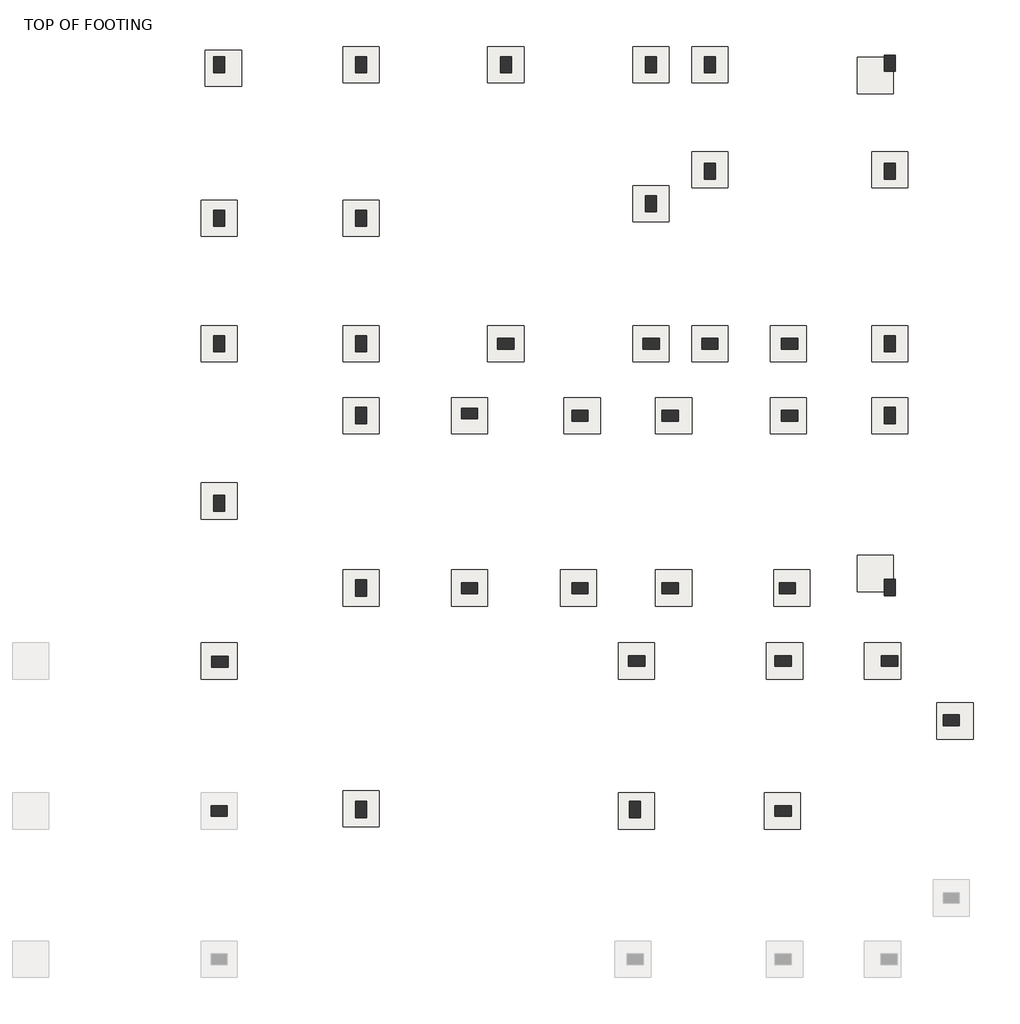
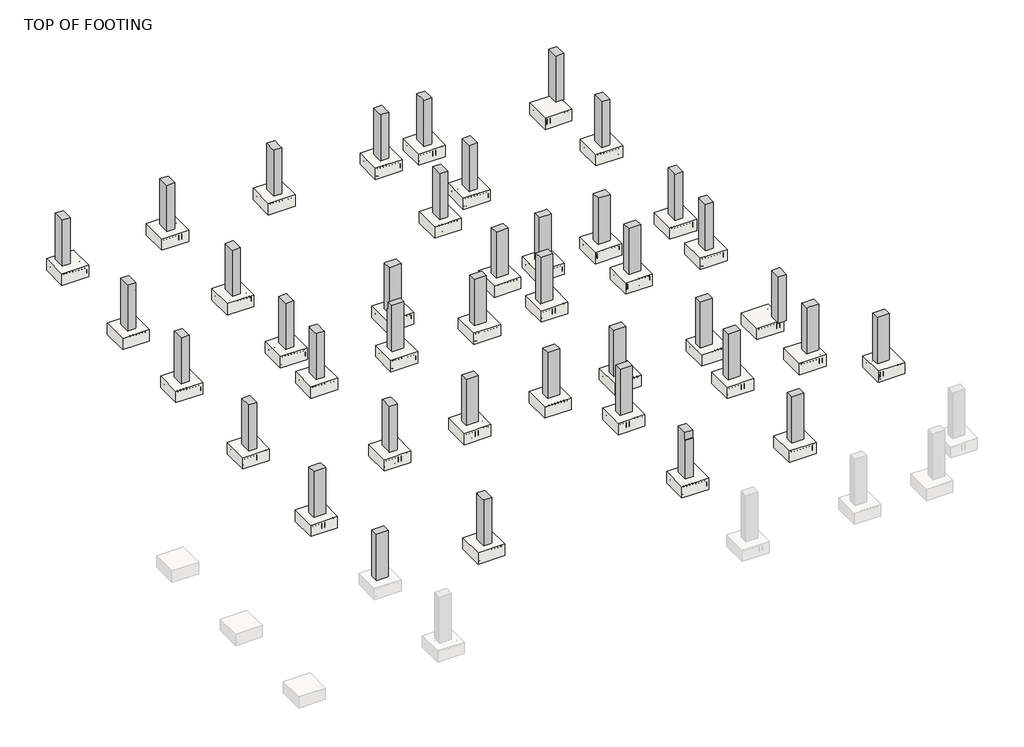
# One storey, part 2 of 20: 40 columns, 39 slabs.
"""IFC4 building model written with IfcOpenShell, lengths in millimetres."""

from ifc_helpers import new_model, si_unit, frame, origin, place, context, project, spatial, polyline, outline, extrude, faceted_brep, transform, mapped, element, save
from components import m_footing_rectangular_4c97ae35

model = new_model("IFC4")

# Units and contexts
model_context = context("Model", 3, world=origin())
ifc_project = project(units=[si_unit("LENGTHUNIT", "METRE", prefix="MILLI")], contexts=[model_context])

# Site, building, storey
site = spatial("IfcSite", under=ifc_project)
building = spatial("IfcBuilding", under=site)
storey = spatial("IfcBuildingStorey", under=building, Name="TOP OF FOOTING", Elevation=-1828.8)

# Columns
placement = place(None, origin())
element("IfcColumn", 1, ObjectType="M_Concrete-Rectangular-Column : 300 x 450mm", at=placement, inside=storey, context=model_context, shape_type="SweptSolid", body=[
    extrude(outline(polyline([(-5591.7865686, 21912.8349362), (-5591.7865686, 21462.8349362), (-5891.7865686, 21462.8349362), (-5891.7865686, 21912.8349362), (-5591.7865686, 21912.8349362)])), frame((0.0, 0.0, -1828.8), z_axis=(0.0, 0.0, 1.0), x_axis=(1.0, 0.0, 0.0)), (0.0, 0.0, 1.0), 1828.8),
])
element("IfcColumn", 2, ObjectType="M_Concrete-Rectangular-Column : 300 x 450mm", at=placement, inside=storey, context=model_context, shape_type="Brep", body=[
    faceted_brep([(-1671.7865686, 21912.8349362, -1828.8), (-1671.7865686, 21462.8349362, -1828.8), (-1971.7865686, 21462.8349362, -1828.8), (-1971.7865686, 21912.8349362, -1828.8), (-1671.7865686, 21912.8349362, 0.0), (-1671.7865686, 21537.8349362, 0.0), (-1671.7865686, 21462.8349362, 0.0), (-1671.7865686, 21462.8349362, -300.0), (-1971.7865686, 21462.8349362, 0.0), (-1971.7865686, 21462.8349362, -300.0), (-1971.7865686, 21912.8349362, 0.0)], [[[0, 1, 2, 3]], [[1, 0, 4, 5, 6, 7]], [[2, 1, 7, 6, 8, 9]], [[3, 2, 9, 8, 10]], [[0, 3, 10, 4]], [[8, 6, 5, 4, 10]]]),
])
element("IfcColumn", 3, ObjectType="M_Concrete-Rectangular-Column : 300 x 450mm", at=placement, inside=storey, context=model_context, shape_type="Brep", body=[
    faceted_brep([(2324.7296816, 21912.8349362, -1828.8), (2324.7296816, 21462.8349362, -1828.8), (2024.7296816, 21462.8349362, -1828.8), (2024.7296816, 21912.8349362, -1828.8), (2324.7296816, 21912.8349362, 0.0), (2324.7296816, 21537.8349362, 0.0), (2324.7296816, 21462.8349362, 0.0), (2324.7296816, 21462.8349362, -300.0), (2024.7296816, 21462.8349362, 0.0), (2024.7296816, 21462.8349362, -300.0), (2024.7296816, 21537.8349362, 0.0), (2024.7296816, 21912.8349362, 0.0)], [[[0, 1, 2, 3]], [[1, 0, 4, 5, 6, 7]], [[2, 1, 7, 6, 8, 9]], [[3, 2, 9, 8, 10, 11]], [[0, 3, 11, 4]], [[8, 6, 5, 4, 11, 10]]]),
])
element("IfcColumn", 4, ObjectType="M_Concrete-Rectangular-Column : 300 x 450mm", at=placement, inside=storey, context=model_context, shape_type="Brep", body=[
    faceted_brep([(6332.5248054, 21912.8349362, -1828.8), (6332.5248054, 21462.8349362, -1828.8), (6032.5248054, 21462.8349362, -1828.8), (6032.5248054, 21912.8349362, -1828.8), (6332.5248054, 21912.8349362, 0.0), (6332.5248054, 21537.8349362, 0.0), (6332.5248054, 21462.8349362, 0.0), (6332.5248054, 21462.8349362, -300.0), (6032.5248054, 21462.8349362, 0.0), (6032.5248054, 21462.8349362, -300.0), (6032.5248054, 21537.8349362, 0.0), (6032.5248054, 21912.8349362, 0.0)], [[[0, 1, 2, 3]], [[1, 0, 4, 5, 6, 7]], [[2, 1, 7, 6, 8, 9]], [[3, 2, 9, 8, 10, 11]], [[0, 3, 11, 4]], [[8, 6, 5, 4, 11, 10]]]),
])
element("IfcColumn", 5, ObjectType="M_Concrete-Rectangular-Column : 300 x 450mm", at=placement, inside=storey, context=model_context, shape_type="Brep", body=[
    faceted_brep([(7956.8679014, 21912.8349362, -1828.8), (7956.8679014, 21462.8349362, -1828.8), (7656.8679014, 21462.8349362, -1828.8), (7656.8679014, 21912.8349362, -1828.8), (7956.8679014, 21912.8349362, 0.0), (7956.8679014, 21537.8349362, 0.0), (7956.8679014, 21462.8349362, 0.0), (7956.8679014, 21462.8349362, -300.0), (7656.8679014, 21462.8349362, 0.0), (7656.8679014, 21462.8349362, -300.0), (7656.8679014, 21537.8349362, 0.0), (7656.8679014, 21912.8349362, 0.0)], [[[0, 1, 2, 3]], [[1, 0, 4, 5, 6, 7]], [[2, 1, 7, 6, 8, 9]], [[3, 2, 9, 8, 10, 11]], [[0, 3, 11, 4]], [[8, 6, 5, 4, 11, 10]]]),
])
element("IfcColumn", 6, ObjectType="M_Concrete-Rectangular-Column : 300 x 450mm", at=placement, inside=storey, context=model_context, shape_type="Brep", body=[
    faceted_brep([(12919.1163908, 21952.8349362, -1828.8), (12919.1163908, 21502.8349362, -1828.8), (12619.1163908, 21502.8349362, -1828.8), (12619.1163908, 21952.8349362, -1828.8), (12919.1163908, 21952.8349362, 0.0), (12919.1163908, 21502.8349362, 0.0), (12619.1163908, 21502.8349362, 0.0), (12619.1163908, 21502.8349362, -300.0), (12619.1163908, 21537.8349362, 0.0), (12619.1163908, 21952.8349362, 0.0)], [[[0, 1, 2, 3]], [[1, 0, 4, 5]], [[2, 1, 5, 6, 7]], [[3, 2, 7, 6, 8, 9]], [[0, 3, 9, 4]], [[5, 4, 9, 8, 6]]]),
])
element("IfcColumn", 7, ObjectType="M_Concrete-Rectangular-Column : 300 x 450mm", at=placement, inside=storey, context=model_context, shape_type="Brep", body=[
    faceted_brep([(12919.1163908, 18974.7148651, -1828.8), (12919.1163908, 18524.7148651, -1828.8), (12619.1163908, 18524.7148651, -1828.8), (12619.1163908, 18974.7148651, -1828.8), (12919.1163908, 18974.7148651, 0.0), (12919.1163908, 18524.7148651, 0.0), (12619.1163908, 18524.7148651, 0.0), (12619.1163908, 18524.7148651, -300.0), (12619.1163908, 18974.7148651, 0.0), (12619.1163908, 18974.7148651, -300.0)], [[[0, 1, 2, 3]], [[1, 0, 4, 5]], [[2, 1, 5, 6, 7]], [[3, 2, 7, 6, 8, 9]], [[0, 3, 9, 8, 4]], [[5, 4, 8, 6]]]),
])
element("IfcColumn", 8, ObjectType="M_Concrete-Rectangular-Column : 300 x 450mm", at=placement, inside=storey, context=model_context, shape_type="Brep", body=[
    faceted_brep([(7956.8679014, 18974.7148651, -1828.8), (7956.8679014, 18524.7148651, -1828.8), (7656.8679014, 18524.7148651, -1828.8), (7656.8679014, 18974.7148651, -1828.8), (7956.8679014, 18974.7148651, -300.0), (7956.8679014, 18974.7148651, 0.0), (7956.8679014, 18524.7148651, 0.0), (7956.8679014, 18524.7148651, -300.0), (7656.8679014, 18524.7148651, 0.0), (7656.8679014, 18524.7148651, -300.0), (7656.8679014, 18974.7148651, 0.0), (7656.8679014, 18974.7148651, -300.0)], [[[0, 1, 2, 3]], [[1, 0, 4, 5, 6, 7]], [[2, 1, 7, 6, 8, 9]], [[3, 2, 9, 8, 10, 11]], [[0, 3, 11, 10, 5, 4]], [[6, 5, 10, 8]]]),
])
element("IfcColumn", 9, ObjectType="M_Concrete-Rectangular-Column : 300 x 450mm", at=placement, inside=storey, context=model_context, shape_type="Brep", body=[
    faceted_brep([(6332.5248054, 18074.7148651, -1828.8), (6332.5248054, 17624.7148651, -1828.8), (6032.5248054, 17624.7148651, -1828.8), (6032.5248054, 18074.7148651, -1828.8), (6332.5248054, 18074.7148651, -300.0), (6332.5248054, 18074.7148651, 0.0), (6332.5248054, 17624.7148651, 0.0), (6332.5248054, 17624.7148651, -300.0), (6032.5248054, 17624.7148651, 0.0), (6032.5248054, 17624.7148651, -300.0), (6032.5248054, 18074.7148651, 0.0), (6032.5248054, 18074.7148651, -300.0)], [[[0, 1, 2, 3]], [[1, 0, 4, 5, 6, 7]], [[2, 1, 7, 6, 8, 9]], [[3, 2, 9, 8, 10, 11]], [[0, 3, 11, 10, 5, 4]], [[6, 5, 10, 8]]]),
])
element("IfcColumn", 10, ObjectType="M_Concrete-Rectangular-Column : 300 x 450mm", at=placement, inside=storey, context=model_context, shape_type="Brep", body=[
    faceted_brep([(-1671.7865686, 17674.7148651, -1828.8), (-1671.7865686, 17224.7148651, -1828.8), (-1971.7865686, 17224.7148651, -1828.8), (-1971.7865686, 17674.7148651, -1828.8), (-1671.7865686, 17674.7148651, -300.0), (-1671.7865686, 17674.7148651, 0.0), (-1671.7865686, 17224.7148651, 0.0), (-1671.7865686, 17224.7148651, -300.0), (-1971.7865686, 17224.7148651, 0.0), (-1971.7865686, 17224.7148651, -300.0), (-1971.7865686, 17674.7148651, 0.0), (-1971.7865686, 17674.7148651, -300.0)], [[[0, 1, 2, 3]], [[1, 0, 4, 5, 6, 7]], [[2, 1, 7, 6, 8, 9]], [[3, 2, 9, 8, 10, 11]], [[0, 3, 11, 10, 5, 4]], [[6, 5, 10, 8]]]),
])
element("IfcColumn", 11, ObjectType="M_Concrete-Rectangular-Column : 300 x 450mm", at=placement, inside=storey, context=model_context, shape_type="SweptSolid", body=[
    extrude(outline(polyline([(-1828.8, -5888.8105653), (-1828.8, -5588.8105653), (-300.0, -5588.8105653), (-300.0, -5591.7865686), (0.0, -5591.7865686), (0.0, -5888.8105653), (-1828.8, -5888.8105653)])), frame((0.0, 17224.7148651, 0.0), z_axis=(0.0, 1.0, 0.0), x_axis=(0.0, 0.0, 1.0)), (0.0, 0.0, 1.0), 450.0),
])
element("IfcColumn", 12, ObjectType="M_Concrete-Rectangular-Column : 300 x 450mm", at=placement, inside=storey, context=model_context, shape_type="Brep", body=[
    faceted_brep([(-5588.8105653, 14212.5179708, -1828.8), (-5588.8105653, 13762.5179708, -1828.8), (-5888.8105653, 13762.5179708, -1828.8), (-5888.8105653, 14212.5179708, -1828.8), (-5588.8105653, 14212.5179708, -300.0), (-5588.8105653, 14212.5179708, 0.0), (-5588.8105653, 13837.5179708, 0.0), (-5588.8105653, 13762.5179708, 0.0), (-5588.8105653, 13762.5179708, -300.0), (-5888.8105653, 13762.5179708, 0.0), (-5888.8105653, 14212.5179708, 0.0), (-5591.7865686, 14212.5179708, 0.0)], [[[0, 1, 2, 3]], [[1, 0, 4, 5, 6, 7, 8]], [[2, 1, 8, 7, 9]], [[3, 2, 9, 10]], [[0, 3, 10, 11, 5, 4]], [[9, 7, 6, 5, 11, 10]]]),
])
element("IfcColumn", 13, ObjectType="M_Concrete-Rectangular-Column : 300 x 450mm", at=placement, inside=storey, context=model_context, shape_type="Brep", body=[
    faceted_brep([(-1671.7865686, 14212.5179708, -1828.8), (-1671.7865686, 13762.5179708, -1828.8), (-1971.7865686, 13762.5179708, -1828.8), (-1971.7865686, 14212.5179708, -1828.8), (-1671.7865686, 14212.5179708, -300.0), (-1671.7865686, 14212.5179708, 0.0), (-1671.7865686, 14137.5179708, 0.0), (-1671.7865686, 13837.5179708, 0.0), (-1671.7865686, 13762.5179708, 0.0), (-1671.7865686, 13762.5179708, -300.0), (-1971.7865686, 13762.5179708, 0.0), (-1971.7865686, 13762.5179708, -300.0), (-1971.7865686, 13837.5179708, 0.0), (-1971.7865686, 14212.5179708, 0.0), (-1971.7865686, 14212.5179708, -300.0)], [[[0, 1, 2, 3]], [[1, 0, 4, 5, 6, 7, 8, 9]], [[2, 1, 9, 8, 10, 11]], [[3, 2, 11, 10, 12, 13, 14]], [[0, 3, 14, 13, 5, 4]], [[10, 8, 7, 6, 5, 13, 12]]]),
])
element("IfcColumn", 14, ObjectType="M_Concrete-Rectangular-Column : 300 x 450mm", at=placement, inside=storey, context=model_context, shape_type="Brep", body=[
    faceted_brep([(1949.7296816, 14137.5179708, -1828.8), (2399.7296816, 14137.5179708, -1828.8), (2399.7296816, 13837.5179708, -1828.8), (1949.7296816, 13837.5179708, -1828.8), (1949.7296816, 14137.5179708, -300.0), (1949.7296816, 14137.5179708, 0.0), (2024.7296816, 14137.5179708, 0.0), (2324.7296816, 14137.5179708, 0.0), (2399.7296816, 14137.5179708, 0.0), (2399.7296816, 14137.5179708, -300.0), (2399.7296816, 13837.5179708, 0.0), (2399.7296816, 13837.5179708, -300.0), (2324.7296816, 13837.5179708, 0.0), (2024.7296816, 13837.5179708, 0.0), (1949.7296816, 13837.5179708, 0.0), (1949.7296816, 13837.5179708, -300.0)], [[[0, 1, 2, 3]], [[1, 0, 4, 5, 6, 7, 8, 9]], [[2, 1, 9, 8, 10, 11]], [[3, 2, 11, 10, 12, 13, 14, 15]], [[0, 3, 15, 14, 5, 4]], [[10, 8, 7, 6, 5, 14, 13, 12]]]),
])
element("IfcColumn", 15, ObjectType="M_Concrete-Rectangular-Column : 300 x 450mm", at=placement, inside=storey, context=model_context, shape_type="Brep", body=[
    faceted_brep([(5957.5248054, 14137.5179708, -1828.8), (6407.5248054, 14137.5179708, -1828.8), (6407.5248054, 13837.5179708, -1828.8), (5957.5248054, 13837.5179708, -1828.8), (5957.5248054, 14137.5179708, -300.0), (5957.5248054, 14137.5179708, 0.0), (6032.5248054, 14137.5179708, 0.0), (6332.5248054, 14137.5179708, 0.0), (6407.5248054, 14137.5179708, 0.0), (6407.5248054, 14137.5179708, -300.0), (6407.5248054, 13837.5179708, 0.0), (6407.5248054, 13837.5179708, -300.0), (6332.5248054, 13837.5179708, 0.0), (6032.5248054, 13837.5179708, 0.0), (5957.5248054, 13837.5179708, 0.0), (5957.5248054, 13837.5179708, -300.0)], [[[0, 1, 2, 3]], [[1, 0, 4, 5, 6, 7, 8, 9]], [[2, 1, 9, 8, 10, 11]], [[3, 2, 11, 10, 12, 13, 14, 15]], [[0, 3, 15, 14, 5, 4]], [[10, 8, 7, 6, 5, 14, 13, 12]]]),
])
element("IfcColumn", 16, ObjectType="M_Concrete-Rectangular-Column : 300 x 450mm", at=placement, inside=storey, context=model_context, shape_type="Brep", body=[
    faceted_brep([(7581.8679014, 14137.5179708, -1828.8), (8031.8679014, 14137.5179708, -1828.8), (8031.8679014, 13837.5179708, -1828.8), (7581.8679014, 13837.5179708, -1828.8), (7581.8679014, 14137.5179708, -300.0), (7581.8679014, 14137.5179708, 0.0), (7656.8679014, 14137.5179708, 0.0), (7956.8679014, 14137.5179708, 0.0), (8031.8679014, 14137.5179708, 0.0), (8031.8679014, 14137.5179708, -300.0), (8031.8679014, 13837.5179708, 0.0), (8031.8679014, 13837.5179708, -300.0), (7956.8679014, 13837.5179708, 0.0), (7656.8679014, 13837.5179708, 0.0), (7581.8679014, 13837.5179708, 0.0), (7581.8679014, 13837.5179708, -300.0)], [[[0, 1, 2, 3]], [[1, 0, 4, 5, 6, 7, 8, 9]], [[2, 1, 9, 8, 10, 11]], [[3, 2, 11, 10, 12, 13, 14, 15]], [[0, 3, 15, 14, 5, 4]], [[10, 8, 7, 6, 5, 14, 13, 12]]]),
])
element("IfcColumn", 17, ObjectType="M_Concrete-Rectangular-Column : 300 x 450mm", at=placement, inside=storey, context=model_context, shape_type="Brep", body=[
    faceted_brep([(9781.8679014, 14137.5179708, -1828.8), (10231.8679014, 14137.5179708, -1828.8), (10231.8679014, 13837.5179708, -1828.8), (9781.8679014, 13837.5179708, -1828.8), (9781.8679014, 14137.5179708, -300.0), (9781.8679014, 14137.5179708, 0.0), (10231.8679014, 14137.5179708, 0.0), (10231.8679014, 14137.5179708, -300.0), (10231.8679014, 13837.5179708, 0.0), (10231.8679014, 13837.5179708, -300.0), (9781.8679014, 13837.5179708, 0.0), (9781.8679014, 13837.5179708, -300.0)], [[[0, 1, 2, 3]], [[1, 0, 4, 5, 6, 7]], [[2, 1, 7, 6, 8, 9]], [[3, 2, 9, 8, 10, 11]], [[0, 3, 11, 10, 5, 4]], [[6, 5, 10, 8]]]),
])
element("IfcColumn", 18, ObjectType="M_Concrete-Rectangular-Column : 300 x 450mm", at=placement, inside=storey, context=model_context, shape_type="Brep", body=[
    faceted_brep([(12619.1163908, 13762.5179708, -1828.8), (12619.1163908, 14212.5179708, -1828.8), (12919.1163908, 14212.5179708, -1828.8), (12919.1163908, 13762.5179708, -1828.8), (12619.1163908, 13762.5179708, -300.0), (12619.1163908, 13762.5179708, 0.0), (12619.1163908, 13837.5179708, 0.0), (12619.1163908, 14137.5179708, 0.0), (12619.1163908, 14212.5179708, 0.0), (12619.1163908, 14212.5179708, -300.0), (12919.1163908, 14212.5179708, 0.0), (12919.1163908, 13762.5179708, 0.0)], [[[0, 1, 2, 3]], [[1, 0, 4, 5, 6, 7, 8, 9]], [[2, 1, 9, 8, 10]], [[3, 2, 10, 11]], [[0, 3, 11, 5, 4]], [[10, 8, 7, 6, 5, 11]]]),
])
element("IfcColumn", 19, ObjectType="M_Concrete-Rectangular-Column : 300 x 450mm", at=placement, inside=storey, context=model_context, shape_type="Brep", body=[
    faceted_brep([(-1971.7865686, 11782.4075451, -1828.8), (-1971.7865686, 12232.4075451, -1828.8), (-1671.7865686, 12232.4075451, -1828.8), (-1671.7865686, 11782.4075451, -1828.8), (-1971.7865686, 11782.4075451, -300.0), (-1971.7865686, 11782.4075451, 0.0), (-1971.7865686, 11857.4075451, 0.0), (-1971.7865686, 12157.4075451, 0.0), (-1971.7865686, 12232.4075451, 0.0), (-1971.7865686, 12232.4075451, -300.0), (-1671.7865686, 12232.4075451, 0.0), (-1671.7865686, 12232.4075451, -300.0), (-1671.7865686, 12157.4075451, 0.0), (-1671.7865686, 11857.4075451, 0.0), (-1671.7865686, 11782.4075451, 0.0), (-1671.7865686, 11782.4075451, -300.0)], [[[0, 1, 2, 3]], [[1, 0, 4, 5, 6, 7, 8, 9]], [[2, 1, 9, 8, 10, 11]], [[3, 2, 11, 10, 12, 13, 14, 15]], [[0, 3, 15, 14, 5, 4]], [[10, 8, 7, 6, 5, 14, 13, 12]]]),
])
element("IfcColumn", 20, ObjectType="M_Concrete-Rectangular-Column : 300 x 450mm", at=placement, inside=storey, context=model_context, shape_type="Brep", body=[
    faceted_brep([(1399.7296816, 11917.4075451, -1828.8), (949.7296816, 11917.4075451, -1828.8), (949.7296816, 12217.4075451, -1828.8), (1399.7296816, 12217.4075451, -1828.8), (1399.7296816, 11917.4075451, -600.0), (1399.7296816, 11917.4075451, 0.0), (949.7296816, 11917.4075451, 0.0), (949.7296816, 11917.4075451, -600.0), (949.7296816, 12157.4075451, 0.0), (949.7296816, 12157.4075451, -300.0), (949.7296816, 12217.4075451, -300.0), (1399.7296816, 12217.4075451, -300.0), (1399.7296816, 12157.4075451, -300.0), (1399.7296816, 12157.4075451, 0.0)], [[[0, 1, 2, 3]], [[1, 0, 4, 5, 6, 7]], [[2, 1, 7, 6, 8, 9, 10]], [[3, 2, 10, 11]], [[0, 3, 11, 12, 13, 5, 4]], [[6, 5, 13, 8]], [[9, 12, 11, 10]], [[12, 9, 8, 13]]]),
])
element("IfcColumn", 21, ObjectType="M_Concrete-Rectangular-Column : 300 x 450mm", at=placement, inside=storey, context=model_context, shape_type="Brep", body=[
    faceted_brep([(4447.5248054, 11857.4075451, -1828.8), (3997.5248054, 11857.4075451, -1828.8), (3997.5248054, 12157.4075451, -1828.8), (4447.5248054, 12157.4075451, -1828.8), (4447.5248054, 11857.4075451, -300.0), (4447.5248054, 11857.4075451, 0.0), (3997.5248054, 11857.4075451, 0.0), (3997.5248054, 11857.4075451, -300.0), (3997.5248054, 12157.4075451, 0.0), (3997.5248054, 12157.4075451, -300.0), (4447.5248054, 12157.4075451, 0.0), (4447.5248054, 12157.4075451, -300.0)], [[[0, 1, 2, 3]], [[1, 0, 4, 5, 6, 7]], [[2, 1, 7, 6, 8, 9]], [[3, 2, 9, 8, 10, 11]], [[0, 3, 11, 10, 5, 4]], [[6, 5, 10, 8]]]),
])
element("IfcColumn", 22, ObjectType="M_Concrete-Rectangular-Column : 300 x 450mm", at=placement, inside=storey, context=model_context, shape_type="Brep", body=[
    faceted_brep([(6931.8679014, 11857.4075451, -1828.8), (6481.8679014, 11857.4075451, -1828.8), (6481.8679014, 12157.4075451, -1828.8), (6931.8679014, 12157.4075451, -1828.8), (6931.8679014, 11857.4075451, -300.0), (6931.8679014, 11857.4075451, 0.0), (6481.8679014, 11857.4075451, 0.0), (6481.8679014, 11857.4075451, -300.0), (6481.8679014, 12157.4075451, 0.0), (6481.8679014, 12157.4075451, -300.0), (6931.8679014, 12157.4075451, 0.0), (6931.8679014, 12157.4075451, -300.0)], [[[0, 1, 2, 3]], [[1, 0, 4, 5, 6, 7]], [[2, 1, 7, 6, 8, 9]], [[3, 2, 9, 8, 10, 11]], [[0, 3, 11, 10, 5, 4]], [[6, 5, 10, 8]]]),
])
element("IfcColumn", 23, ObjectType="M_Concrete-Rectangular-Column : 300 x 450mm", at=placement, inside=storey, context=model_context, shape_type="Brep", body=[
    faceted_brep([(10231.8679014, 11857.4075451, -1828.8), (9781.8679014, 11857.4075451, -1828.8), (9781.8679014, 12157.4075451, -1828.8), (10231.8679014, 12157.4075451, -1828.8), (10231.8679014, 11857.4075451, -300.0), (10231.8679014, 11857.4075451, 0.0), (9781.8679014, 11857.4075451, 0.0), (9781.8679014, 11857.4075451, -300.0), (9781.8679014, 12157.4075451, 0.0), (9781.8679014, 12157.4075451, -300.0), (10231.8679014, 12157.4075451, 0.0), (10231.8679014, 12157.4075451, -300.0)], [[[0, 1, 2, 3]], [[1, 0, 4, 5, 6, 7]], [[2, 1, 7, 6, 8, 9]], [[3, 2, 9, 8, 10, 11]], [[0, 3, 11, 10, 5, 4]], [[6, 5, 10, 8]]]),
])
element("IfcColumn", 24, ObjectType="M_Concrete-Rectangular-Column : 300 x 450mm", at=placement, inside=storey, context=model_context, shape_type="Brep", body=[
    faceted_brep([(12919.1163908, 12232.4075451, -1828.8), (12919.1163908, 11782.4075451, -1828.8), (12619.1163908, 11782.4075451, -1828.8), (12619.1163908, 12232.4075451, -1828.8), (12919.1163908, 12232.4075451, 0.0), (12919.1163908, 11782.4075451, 0.0), (12619.1163908, 11782.4075451, 0.0), (12619.1163908, 12157.4075451, 0.0), (12619.1163908, 12232.4075451, 0.0), (12619.1163908, 12232.4075451, -300.0)], [[[0, 1, 2, 3]], [[1, 0, 4, 5]], [[2, 1, 5, 6]], [[3, 2, 6, 7, 8, 9]], [[0, 3, 9, 8, 4]], [[5, 4, 8, 7, 6]]]),
])
element("IfcColumn", 25, ObjectType="M_Concrete-Rectangular-Column : 300 x 450mm", at=placement, inside=storey, context=model_context, shape_type="Brep", body=[
    faceted_brep([(-5888.8105653, 9367.5252033, -1828.8), (-5888.8105653, 9817.5252033, -1828.8), (-5588.8105653, 9817.5252033, -1828.8), (-5588.8105653, 9367.5252033, -1828.8), (-5888.8105653, 9367.5252033, 0.0), (-5888.8105653, 9817.5252033, 0.0), (-5588.8105653, 9817.5252033, 0.0), (-5588.8105653, 9817.5252033, -300.0), (-5588.8105653, 9367.5252033, 0.0), (-5588.8105653, 9367.5252033, -300.0)], [[[0, 1, 2, 3]], [[1, 0, 4, 5]], [[2, 1, 5, 6, 7]], [[3, 2, 7, 6, 8, 9]], [[0, 3, 9, 8, 4]], [[5, 4, 8, 6]]]),
])
element("IfcColumn", 26, ObjectType="M_Concrete-Rectangular-Column : 300 x 450mm", at=placement, inside=storey, context=model_context, shape_type="Brep", body=[
    faceted_brep([(-1971.7865686, 7024.7076276, -1828.8), (-1971.7865686, 7474.7076276, -1828.8), (-1671.7865686, 7474.7076276, -1828.8), (-1671.7865686, 7024.7076276, -1828.8), (-1971.7865686, 7024.7076276, -300.0), (-1971.7865686, 7024.7076276, 0.0), (-1971.7865686, 7099.7076276, 0.0), (-1971.7865686, 7399.7076276, 0.0), (-1971.7865686, 7474.7076276, 0.0), (-1971.7865686, 7474.7076276, -300.0), (-1671.7865686, 7474.7076276, 0.0), (-1671.7865686, 7474.7076276, -300.0), (-1671.7865686, 7399.7076276, 0.0), (-1671.7865686, 7099.7076276, 0.0), (-1671.7865686, 7024.7076276, 0.0), (-1671.7865686, 7024.7076276, -300.0)], [[[0, 1, 2, 3]], [[1, 0, 4, 5, 6, 7, 8, 9]], [[2, 1, 9, 8, 10, 11]], [[3, 2, 11, 10, 12, 13, 14, 15]], [[0, 3, 15, 14, 5, 4]], [[10, 8, 7, 6, 5, 14, 13, 12]]]),
])
element("IfcColumn", 27, ObjectType="M_Concrete-Rectangular-Column : 300 x 450mm", at=placement, inside=storey, context=model_context, shape_type="Brep", body=[
    faceted_brep([(1399.7296816, 7099.7076276, -1828.8), (949.7296816, 7099.7076276, -1828.8), (949.7296816, 7399.7076276, -1828.8), (1399.7296816, 7399.7076276, -1828.8), (1399.7296816, 7099.7076276, -300.0), (1399.7296816, 7099.7076276, 0.0), (949.7296816, 7099.7076276, 0.0), (949.7296816, 7099.7076276, -300.0), (949.7296816, 7399.7076276, 0.0), (949.7296816, 7399.7076276, -300.0), (1399.7296816, 7399.7076276, 0.0), (1399.7296816, 7399.7076276, -300.0)], [[[0, 1, 2, 3]], [[1, 0, 4, 5, 6, 7]], [[2, 1, 7, 6, 8, 9]], [[3, 2, 9, 8, 10, 11]], [[0, 3, 11, 10, 5, 4]], [[6, 5, 10, 8]]]),
])
element("IfcColumn", 28, ObjectType="M_Concrete-Rectangular-Column : 300 x 450mm", at=placement, inside=storey, context=model_context, shape_type="Brep", body=[
    faceted_brep([(4447.5248054, 7099.7076276, -1828.8), (3997.5248054, 7099.7076276, -1828.8), (3997.5248054, 7399.7076276, -1828.8), (4447.5248054, 7399.7076276, -1828.8), (4447.5248054, 7099.7076276, -300.0), (4447.5248054, 7099.7076276, 0.0), (3997.5248054, 7099.7076276, 0.0), (3997.5248054, 7099.7076276, -300.0), (3997.5248054, 7399.7076276, 0.0), (3997.5248054, 7399.7076276, -300.0), (4447.5248054, 7399.7076276, 0.0), (4447.5248054, 7399.7076276, -300.0)], [[[0, 1, 2, 3]], [[1, 0, 4, 5, 6, 7]], [[2, 1, 7, 6, 8, 9]], [[3, 2, 9, 8, 10, 11]], [[0, 3, 11, 10, 5, 4]], [[6, 5, 10, 8]]]),
])
element("IfcColumn", 29, ObjectType="M_Concrete-Rectangular-Column : 300 x 450mm", at=placement, inside=storey, context=model_context, shape_type="Brep", body=[
    faceted_brep([(6931.8679014, 7099.7076276, -1828.8), (6481.8679014, 7099.7076276, -1828.8), (6481.8679014, 7399.7076276, -1828.8), (6931.8679014, 7399.7076276, -1828.8), (6931.8679014, 7099.7076276, -300.0), (6931.8679014, 7099.7076276, 0.0), (6481.8679014, 7099.7076276, 0.0), (6481.8679014, 7099.7076276, -300.0), (6481.8679014, 7399.7076276, 0.0), (6481.8679014, 7399.7076276, -300.0), (6931.8679014, 7399.7076276, 0.0), (6931.8679014, 7399.7076276, -300.0)], [[[0, 1, 2, 3]], [[1, 0, 4, 5, 6, 7]], [[2, 1, 7, 6, 8, 9]], [[3, 2, 9, 8, 10, 11]], [[0, 3, 11, 10, 5, 4]], [[6, 5, 10, 8]]]),
])
element("IfcColumn", 30, ObjectType="M_Concrete-Rectangular-Column : 300 x 450mm", at=placement, inside=storey, context=model_context, shape_type="Brep", body=[
    faceted_brep([(10171.8679014, 7099.7076276, -1828.8), (9721.8679014, 7099.7076276, -1828.8), (9721.8679014, 7399.7076276, -1828.8), (10171.8679014, 7399.7076276, -1828.8), (10171.8679014, 7099.7076276, -300.0), (10171.8679014, 7099.7076276, 0.0), (9721.8679014, 7099.7076276, 0.0), (9721.8679014, 7099.7076276, -300.0), (9721.8679014, 7399.7076276, 0.0), (9721.8679014, 7399.7076276, -300.0), (10171.8679014, 7399.7076276, 0.0), (10171.8679014, 7399.7076276, -300.0)], [[[0, 1, 2, 3]], [[1, 0, 4, 5, 6, 7]], [[2, 1, 7, 6, 8, 9]], [[3, 2, 9, 8, 10, 11]], [[0, 3, 11, 10, 5, 4]], [[6, 5, 10, 8]]]),
])
element("IfcColumn", 31, ObjectType="M_Concrete-Rectangular-Column : 300 x 450mm", at=placement, inside=storey, context=model_context, shape_type="SweptSolid", body=[
    extrude(outline(polyline([(12919.1163908, 7494.7076276), (12919.1163908, 7044.7076276), (12619.1163908, 7044.7076276), (12619.1163908, 7494.7076276), (12919.1163908, 7494.7076276)])), frame((0.0, 0.0, -1828.8), z_axis=(0.0, 0.0, 1.0), x_axis=(1.0, 0.0, 0.0)), (0.0, 0.0, 1.0), 1828.8),
])
element("IfcColumn", 32, ObjectType="M_Concrete-Rectangular-Column : 300 x 450mm", at=placement, inside=storey, context=model_context, shape_type="Brep", body=[
    faceted_brep([(-5943.8105653, 5367.6057249, -1828.8), (-5493.8105653, 5367.6057249, -1828.8), (-5493.8105653, 5067.6057249, -1828.8), (-5943.8105653, 5067.6057249, -1828.8), (-5943.8105653, 5367.6057249, 0.0), (-5588.8105653, 5367.6057249, 0.0), (-5493.8105653, 5367.6057249, 0.0), (-5493.8105653, 5367.6057249, -300.0), (-5493.8105653, 5067.6057249, 0.0), (-5493.8105653, 5067.6057249, -300.0), (-5943.8105653, 5067.6057249, 0.0), (-5943.8105653, 5067.6057249, -300.0)], [[[0, 1, 2, 3]], [[1, 0, 4, 5, 6, 7]], [[2, 1, 7, 6, 8, 9]], [[3, 2, 9, 8, 10, 11]], [[0, 3, 11, 10, 4]], [[8, 6, 5, 4, 10]]]),
])
element("IfcColumn", 33, ObjectType="M_Concrete-Rectangular-Column : 300 x 450mm", at=placement, inside=storey, context=model_context, shape_type="Brep", body=[
    faceted_brep([(5557.5248054, 5387.6057249, -1828.8), (6007.5248054, 5387.6057249, -1828.8), (6007.5248054, 5087.6057249, -1828.8), (5557.5248054, 5087.6057249, -1828.8), (5557.5248054, 5387.6057249, -300.0), (5557.5248054, 5387.6057249, 0.0), (6007.5248054, 5387.6057249, 0.0), (6007.5248054, 5387.6057249, -300.0), (6007.5248054, 5087.6057249, 0.0), (6007.5248054, 5087.6057249, -300.0), (5557.5248054, 5087.6057249, 0.0), (5557.5248054, 5087.6057249, -300.0)], [[[0, 1, 2, 3]], [[1, 0, 4, 5, 6, 7]], [[2, 1, 7, 6, 8, 9]], [[3, 2, 9, 8, 10, 11]], [[0, 3, 11, 10, 5, 4]], [[6, 5, 10, 8]]]),
])
element("IfcColumn", 34, ObjectType="M_Concrete-Rectangular-Column : 300 x 450mm", at=placement, inside=storey, context=model_context, shape_type="Brep", body=[
    faceted_brep([(9601.8679014, 5387.6057249, -1828.8), (10051.8679014, 5387.6057249, -1828.8), (10051.8679014, 5087.6057249, -1828.8), (9601.8679014, 5087.6057249, -1828.8), (9601.8679014, 5387.6057249, -300.0), (9601.8679014, 5387.6057249, 0.0), (10051.8679014, 5387.6057249, 0.0), (10051.8679014, 5387.6057249, -300.0), (10051.8679014, 5087.6057249, 0.0), (10051.8679014, 5087.6057249, -300.0), (9601.8679014, 5087.6057249, 0.0), (9601.8679014, 5087.6057249, -300.0)], [[[0, 1, 2, 3]], [[1, 0, 4, 5, 6, 7]], [[2, 1, 7, 6, 8, 9]], [[3, 2, 9, 8, 10, 11]], [[0, 3, 11, 10, 5, 4]], [[6, 5, 10, 8]]]),
])
element("IfcColumn", 35, ObjectType="M_Concrete-Rectangular-Column : 300 x 450mm", at=placement, inside=storey, context=model_context, shape_type="Brep", body=[
    faceted_brep([(12541.8679014, 5387.6057249, -1828.8), (12991.8679014, 5387.6057249, -1828.8), (12991.8679014, 5087.6057249, -1828.8), (12541.8679014, 5087.6057249, -1828.8), (12541.8679014, 5387.6057249, -300.0), (12541.8679014, 5387.6057249, 0.0), (12616.8679014, 5387.6057249, 0.0), (12991.8679014, 5387.6057249, 0.0), (12991.8679014, 5087.6057249, 0.0), (12616.8679014, 5087.6057249, 0.0), (12541.8679014, 5087.6057249, 0.0), (12541.8679014, 5087.6057249, -300.0)], [[[0, 1, 2, 3]], [[1, 0, 4, 5, 6, 7]], [[2, 1, 7, 8]], [[3, 2, 8, 9, 10, 11]], [[0, 3, 11, 10, 5, 4]], [[8, 7, 6, 5, 10, 9]]]),
])
element("IfcColumn", 36, ObjectType="M_Concrete-Rectangular-Column : 300 x 450mm", at=placement, inside=storey, context=model_context, shape_type="Brep", body=[
    faceted_brep([(-5513.8105653, 951.1713929, -1828.8), (-5963.8105653, 951.1713929, -1828.8), (-5963.8105653, 1251.1713929, -1828.8), (-5513.8105653, 1251.1713929, -1828.8), (-5513.8105653, 951.1713929, -300.0), (-5513.8105653, 951.1713929, 0.0), (-5963.8105653, 951.1713929, 0.0), (-5963.8105653, 951.1713929, -300.0), (-5963.8105653, 1251.1713929, 0.0), (-5963.8105653, 1251.1713929, -300.0), (-5513.8105653, 1251.1713929, 0.0), (-5513.8105653, 1251.1713929, -300.0)], [[[0, 1, 2, 3]], [[1, 0, 4, 5, 6, 7]], [[2, 1, 7, 6, 8, 9]], [[3, 2, 9, 8, 10, 11]], [[0, 3, 11, 10, 5, 4]], [[6, 5, 10, 8]]]),
])
element("IfcColumn", 37, ObjectType="M_Concrete-Rectangular-Column : 300 x 450mm", at=placement, inside=storey, context=model_context, shape_type="Brep", body=[
    faceted_brep([(-1671.7865686, 1366.1713929, -1828.8), (-1671.7865686, 916.1713929, -1828.8), (-1971.7865686, 916.1713929, -1828.8), (-1971.7865686, 1366.1713929, -1828.8), (-1671.7865686, 1366.1713929, -300.0), (-1671.7865686, 1366.1713929, 0.0), (-1671.7865686, 1251.1713929, 0.0), (-1671.7865686, 951.1713929, 0.0), (-1671.7865686, 916.1713929, 0.0), (-1671.7865686, 916.1713929, -300.0), (-1971.7865686, 916.1713929, 0.0), (-1971.7865686, 916.1713929, -300.0), (-1971.7865686, 951.1713929, 0.0), (-1971.7865686, 1251.1713929, 0.0), (-1971.7865686, 1366.1713929, 0.0), (-1971.7865686, 1366.1713929, -300.0)], [[[0, 1, 2, 3]], [[1, 0, 4, 5, 6, 7, 8, 9]], [[2, 1, 9, 8, 10, 11]], [[3, 2, 11, 10, 12, 13, 14, 15]], [[0, 3, 15, 14, 5, 4]], [[10, 8, 7, 6, 5, 14, 13, 12]]]),
])
element("IfcColumn", 38, ObjectType="M_Concrete-Rectangular-Column : 300 x 450mm", at=placement, inside=storey, context=model_context, shape_type="Brep", body=[
    faceted_brep([(5892.5248054, 1366.1713929, -1828.8), (5892.5248054, 916.1713929, -1828.8), (5592.5248054, 916.1713929, -1828.8), (5592.5248054, 1366.1713929, -1828.8), (5892.5248054, 1366.1713929, -300.0), (5892.5248054, 1366.1713929, 0.0), (5892.5248054, 1251.1713929, 0.0), (5892.5248054, 951.1713929, 0.0), (5892.5248054, 951.1713929, -300.0), (5892.5248054, 916.1713929, -300.0), (5592.5248054, 916.1713929, -300.0), (5592.5248054, 951.1713929, -300.0), (5592.5248054, 951.1713929, 0.0), (5592.5248054, 1251.1713929, 0.0), (5592.5248054, 1366.1713929, 0.0), (5592.5248054, 1366.1713929, -300.0)], [[[0, 1, 2, 3]], [[1, 0, 4, 5, 6, 7, 8, 9]], [[2, 1, 9, 10]], [[3, 2, 10, 11, 12, 13, 14, 15]], [[0, 3, 15, 14, 5, 4]], [[5, 14, 13, 12, 7, 6]], [[8, 11, 10, 9]], [[11, 8, 7, 12]]]),
])
element("IfcColumn", 39, ObjectType="M_Concrete-Rectangular-Column : 300 x 450mm", at=placement, inside=storey, context=model_context, shape_type="Brep", body=[
    faceted_brep([(9601.8679014, 1251.1713929, -1828.8), (10051.8679014, 1251.1713929, -1828.8), (10051.8679014, 951.1713929, -1828.8), (9601.8679014, 951.1713929, -1828.8), (9601.8679014, 1251.1713929, -300.0), (9601.8679014, 1251.1713929, 0.0), (10051.8679014, 1251.1713929, 0.0), (10051.8679014, 1251.1713929, -300.0), (10051.8679014, 951.1713929, 0.0), (10051.8679014, 951.1713929, -300.0), (9601.8679014, 951.1713929, 0.0), (9601.8679014, 951.1713929, -300.0)], [[[0, 1, 2, 3]], [[1, 0, 4, 5, 6, 7]], [[2, 1, 7, 6, 8, 9]], [[3, 2, 9, 8, 10, 11]], [[0, 3, 11, 10, 5, 4]], [[6, 5, 10, 8]]]),
])
element("IfcColumn", 40, ObjectType="M_Concrete-Rectangular-Column : 300 x 450mm", at=placement, inside=storey, context=model_context, shape_type="SweptSolid", body=[
    extrude(outline(polyline([(14244.1163908, 3755.7536525), (14694.1163908, 3755.7536525), (14694.1163908, 3455.7536525), (14244.1163908, 3455.7536525), (14244.1163908, 3755.7536525)])), frame((0.0, 0.0, -1828.8), z_axis=(0.0, 0.0, 1.0), x_axis=(1.0, 0.0, 0.0)), (0.0, 0.0, 1.0), 1828.8),
])

# Slabs
m_footing_rectangular_shape = m_footing_rectangular_4c97ae35(model_context)
element("IfcSlab", 41, ObjectType="M_Footing-Rectangular", at=placement, inside=storey, context=model_context, shape_type="MappedRepresentation", body=[
    mapped(m_footing_rectangular_shape, transform((-5621.7865686, 21587.8349362, -1828.8), x_axis=(1.0, 0.0, 0.0), y_axis=(0.0, 1.0, 0.0), z_axis=(0.0, 0.0, 1.0))),
])
element("IfcSlab", 42, ObjectType="M_Footing-Rectangular", at=placement, inside=storey, context=model_context, shape_type="MappedRepresentation", body=[
    mapped(m_footing_rectangular_shape, transform((-1821.7865686, 21687.8349362, -1828.8), x_axis=(1.0, 0.0, 0.0), y_axis=(0.0, 1.0, 0.0), z_axis=(0.0, 0.0, 1.0))),
])
element("IfcSlab", 43, ObjectType="M_Footing-Rectangular", at=placement, inside=storey, context=model_context, shape_type="MappedRepresentation", body=[
    mapped(m_footing_rectangular_shape, transform((2174.7296816, 21687.8349362, -1828.8), x_axis=(1.0, 0.0, 0.0), y_axis=(0.0, 1.0, 0.0), z_axis=(0.0, 0.0, 1.0))),
])
element("IfcSlab", 44, ObjectType="M_Footing-Rectangular", at=placement, inside=storey, context=model_context, shape_type="MappedRepresentation", body=[
    mapped(m_footing_rectangular_shape, transform((6182.5248054, 21687.8349362, -1828.8), x_axis=(1.0, 0.0, 0.0), y_axis=(0.0, 1.0, 0.0), z_axis=(0.0, 0.0, 1.0))),
])
element("IfcSlab", 45, ObjectType="M_Footing-Rectangular", at=placement, inside=storey, context=model_context, shape_type="MappedRepresentation", body=[
    mapped(m_footing_rectangular_shape, transform((7806.8679014, 21687.8349362, -1828.8), x_axis=(1.0, 0.0, 0.0), y_axis=(0.0, 1.0, 0.0), z_axis=(0.0, 0.0, 1.0))),
])
element("IfcSlab", 46, ObjectType="M_Footing-Rectangular", at=placement, inside=storey, context=model_context, shape_type="MappedRepresentation", body=[
    mapped(m_footing_rectangular_shape, transform((12369.1163908, 21387.8349362, -1828.8), x_axis=(1.0, 0.0, 0.0), y_axis=(0.0, 1.0, 0.0), z_axis=(0.0, 0.0, 1.0))),
])
element("IfcSlab", 47, ObjectType="M_Footing-Rectangular", at=placement, inside=storey, context=model_context, shape_type="MappedRepresentation", body=[
    mapped(m_footing_rectangular_shape, transform((12769.1163908, 18787.8349362, -1828.8), x_axis=(1.0, 0.0, 0.0), y_axis=(0.0, 1.0, 0.0), z_axis=(0.0, 0.0, 1.0))),
])
element("IfcSlab", 48, ObjectType="M_Footing-Rectangular", at=placement, inside=storey, context=model_context, shape_type="MappedRepresentation", body=[
    mapped(m_footing_rectangular_shape, transform((7806.8679014, 18787.8349362, -1828.8), x_axis=(1.0, 0.0, 0.0), y_axis=(0.0, 1.0, 0.0), z_axis=(0.0, 0.0, 1.0))),
])
element("IfcSlab", 49, ObjectType="M_Footing-Rectangular", at=placement, inside=storey, context=model_context, shape_type="MappedRepresentation", body=[
    mapped(m_footing_rectangular_shape, transform((6182.5248054, 17849.7148651, -1828.8), x_axis=(1.0, 0.0, 0.0), y_axis=(0.0, 1.0, 0.0), z_axis=(0.0, 0.0, 1.0))),
])
element("IfcSlab", 50, ObjectType="M_Footing-Rectangular", at=placement, inside=storey, context=model_context, shape_type="MappedRepresentation", body=[
    mapped(m_footing_rectangular_shape, transform((-1821.7865686, 17449.7148651, -1828.8), x_axis=(1.0, 0.0, 0.0), y_axis=(0.0, 1.0, 0.0), z_axis=(0.0, 0.0, 1.0))),
])
element("IfcSlab", 51, ObjectType="M_Footing-Rectangular", at=placement, inside=storey, context=model_context, shape_type="MappedRepresentation", body=[
    mapped(m_footing_rectangular_shape, transform((-5738.8105653, 17449.7148651, -1828.8), x_axis=(1.0, 0.0, 0.0), y_axis=(0.0, 1.0, 0.0), z_axis=(0.0, 0.0, 1.0))),
])
element("IfcSlab", 52, ObjectType="M_Footing-Rectangular", at=placement, inside=storey, context=model_context, shape_type="MappedRepresentation", body=[
    mapped(m_footing_rectangular_shape, transform((-5738.8105653, 13987.5179708, -1828.8), x_axis=(1.0, 0.0, 0.0), y_axis=(0.0, 1.0, 0.0), z_axis=(0.0, 0.0, 1.0))),
])
element("IfcSlab", 53, ObjectType="M_Footing-Rectangular", at=placement, inside=storey, context=model_context, shape_type="MappedRepresentation", body=[
    mapped(m_footing_rectangular_shape, transform((-1821.7865686, 13987.5179708, -1828.8), x_axis=(1.0, 0.0, 0.0), y_axis=(0.0, 1.0, 0.0), z_axis=(0.0, 0.0, 1.0))),
])
element("IfcSlab", 54, ObjectType="M_Footing-Rectangular", at=placement, inside=storey, context=model_context, shape_type="MappedRepresentation", body=[
    mapped(m_footing_rectangular_shape, transform((2174.7296816, 13987.5179708, -1828.8), x_axis=(1.0, 0.0, 0.0), y_axis=(0.0, 1.0, 0.0), z_axis=(0.0, 0.0, 1.0))),
])
element("IfcSlab", 55, ObjectType="M_Footing-Rectangular", at=placement, inside=storey, context=model_context, shape_type="MappedRepresentation", body=[
    mapped(m_footing_rectangular_shape, transform((6182.5248054, 13987.5179708, -1828.8), x_axis=(1.0, 0.0, 0.0), y_axis=(0.0, 1.0, 0.0), z_axis=(0.0, 0.0, 1.0))),
])
element("IfcSlab", 56, ObjectType="M_Footing-Rectangular", at=placement, inside=storey, context=model_context, shape_type="MappedRepresentation", body=[
    mapped(m_footing_rectangular_shape, transform((7806.8679014, 13987.5179708, -1828.8), x_axis=(1.0, 0.0, 0.0), y_axis=(0.0, 1.0, 0.0), z_axis=(0.0, 0.0, 1.0))),
])
element("IfcSlab", 57, ObjectType="M_Footing-Rectangular", at=placement, inside=storey, context=model_context, shape_type="MappedRepresentation", body=[
    mapped(m_footing_rectangular_shape, transform((9969.1163908, 13987.5179708, -1828.8), x_axis=(1.0, 0.0, 0.0), y_axis=(0.0, 1.0, 0.0), z_axis=(0.0, 0.0, 1.0))),
])
element("IfcSlab", 58, ObjectType="M_Footing-Rectangular", at=placement, inside=storey, context=model_context, shape_type="MappedRepresentation", body=[
    mapped(m_footing_rectangular_shape, transform((12769.1163908, 13987.5179708, -1828.8), x_axis=(1.0, 0.0, 0.0), y_axis=(0.0, 1.0, 0.0), z_axis=(0.0, 0.0, 1.0))),
])
element("IfcSlab", 59, ObjectType="M_Footing-Rectangular", at=placement, inside=storey, context=model_context, shape_type="MappedRepresentation", body=[
    mapped(m_footing_rectangular_shape, transform((12769.1163908, 12007.4075451, -1828.8), x_axis=(1.0, 0.0, 0.0), y_axis=(0.0, 1.0, 0.0), z_axis=(0.0, 0.0, 1.0))),
])
element("IfcSlab", 60, ObjectType="M_Footing-Rectangular", at=placement, inside=storey, context=model_context, shape_type="MappedRepresentation", body=[
    mapped(m_footing_rectangular_shape, transform((9969.1163908, 12007.4075451, -1828.8), x_axis=(1.0, 0.0, 0.0), y_axis=(0.0, 1.0, 0.0), z_axis=(0.0, 0.0, 1.0))),
])
element("IfcSlab", 61, ObjectType="M_Footing-Rectangular", at=placement, inside=storey, context=model_context, shape_type="MappedRepresentation", body=[
    mapped(m_footing_rectangular_shape, transform((6806.8679014, 12007.4075451, -1828.8), x_axis=(1.0, 0.0, 0.0), y_axis=(0.0, 1.0, 0.0), z_axis=(0.0, 0.0, 1.0))),
])
element("IfcSlab", 62, ObjectType="M_Footing-Rectangular", at=placement, inside=storey, context=model_context, shape_type="MappedRepresentation", body=[
    mapped(m_footing_rectangular_shape, transform((4282.5248054, 12007.4075451, -1828.8), x_axis=(1.0, 0.0, 0.0), y_axis=(0.0, 1.0, 0.0), z_axis=(0.0, 0.0, 1.0))),
])
element("IfcSlab", 63, ObjectType="M_Footing-Rectangular", at=placement, inside=storey, context=model_context, shape_type="MappedRepresentation", body=[
    mapped(m_footing_rectangular_shape, transform((1174.7296816, 12007.4075451, -1828.8), x_axis=(1.0, 0.0, 0.0), y_axis=(0.0, 1.0, 0.0), z_axis=(0.0, 0.0, 1.0))),
])
element("IfcSlab", 64, ObjectType="M_Footing-Rectangular", at=placement, inside=storey, context=model_context, shape_type="MappedRepresentation", body=[
    mapped(m_footing_rectangular_shape, transform((-1821.7865686, 12007.4075451, -1828.8), x_axis=(1.0, 0.0, 0.0), y_axis=(0.0, 1.0, 0.0), z_axis=(0.0, 0.0, 1.0))),
])
element("IfcSlab", 65, ObjectType="M_Footing-Rectangular", at=placement, inside=storey, context=model_context, shape_type="MappedRepresentation", body=[
    mapped(m_footing_rectangular_shape, transform((-5738.8105653, 9649.7076276, -1828.8), x_axis=(1.0, 0.0, 0.0), y_axis=(0.0, 1.0, 0.0), z_axis=(0.0, 0.0, 1.0))),
])
element("IfcSlab", 66, ObjectType="M_Footing-Rectangular", at=placement, inside=storey, context=model_context, shape_type="MappedRepresentation", body=[
    mapped(m_footing_rectangular_shape, transform((-1821.7865686, 7249.7076276, -1828.8), x_axis=(1.0, 0.0, 0.0), y_axis=(0.0, 1.0, 0.0), z_axis=(0.0, 0.0, 1.0))),
])
element("IfcSlab", 67, ObjectType="M_Footing-Rectangular", at=placement, inside=storey, context=model_context, shape_type="MappedRepresentation", body=[
    mapped(m_footing_rectangular_shape, transform((1174.7296816, 7249.7076276, -1828.8), x_axis=(1.0, 0.0, 0.0), y_axis=(0.0, 1.0, 0.0), z_axis=(0.0, 0.0, 1.0))),
])
element("IfcSlab", 68, ObjectType="M_Footing-Rectangular", at=placement, inside=storey, context=model_context, shape_type="MappedRepresentation", body=[
    mapped(m_footing_rectangular_shape, transform((4182.5248054, 7249.7076276, -1828.8), x_axis=(1.0, 0.0, 0.0), y_axis=(0.0, 1.0, 0.0), z_axis=(0.0, 0.0, 1.0))),
])
element("IfcSlab", 69, ObjectType="M_Footing-Rectangular", at=placement, inside=storey, context=model_context, shape_type="MappedRepresentation", body=[
    mapped(m_footing_rectangular_shape, transform((6806.8679014, 7249.7076276, -1828.8), x_axis=(1.0, 0.0, 0.0), y_axis=(0.0, 1.0, 0.0), z_axis=(0.0, 0.0, 1.0))),
])
element("IfcSlab", 70, ObjectType="M_Footing-Rectangular", at=placement, inside=storey, context=model_context, shape_type="MappedRepresentation", body=[
    mapped(m_footing_rectangular_shape, transform((10069.1163908, 7249.7076276, -1828.8), x_axis=(1.0, 0.0, 0.0), y_axis=(0.0, 1.0, 0.0), z_axis=(0.0, 0.0, 1.0))),
])
element("IfcSlab", 71, ObjectType="M_Footing-Rectangular", at=placement, inside=storey, context=model_context, shape_type="MappedRepresentation", body=[
    mapped(m_footing_rectangular_shape, transform((12369.1163908, 7649.7076276, -1828.8), x_axis=(1.0, 0.0, 0.0), y_axis=(0.0, 1.0, 0.0), z_axis=(0.0, 0.0, 1.0))),
])
element("IfcSlab", 72, ObjectType="M_Footing-Rectangular", at=placement, inside=storey, context=model_context, shape_type="MappedRepresentation", body=[
    mapped(m_footing_rectangular_shape, transform((-5738.8105653, 5237.6057249, -1828.8), x_axis=(1.0, 0.0, 0.0), y_axis=(0.0, 1.0, 0.0), z_axis=(0.0, 0.0, 1.0))),
])
element("IfcSlab", 73, ObjectType="M_Footing-Rectangular", at=placement, inside=storey, context=model_context, shape_type="MappedRepresentation", body=[
    mapped(m_footing_rectangular_shape, transform((5782.5248054, 5237.6057249, -1828.8), x_axis=(1.0, 0.0, 0.0), y_axis=(0.0, 1.0, 0.0), z_axis=(0.0, 0.0, 1.0))),
])
element("IfcSlab", 74, ObjectType="M_Footing-Rectangular", at=placement, inside=storey, context=model_context, shape_type="MappedRepresentation", body=[
    mapped(m_footing_rectangular_shape, transform((9869.1163908, 5237.6057249, -1828.8), x_axis=(1.0, 0.0, 0.0), y_axis=(0.0, 1.0, 0.0), z_axis=(0.0, 0.0, 1.0))),
])
element("IfcSlab", 75, ObjectType="M_Footing-Rectangular", at=placement, inside=storey, context=model_context, shape_type="MappedRepresentation", body=[
    mapped(m_footing_rectangular_shape, transform((12569.1163908, 5237.6057249, -1828.8), x_axis=(1.0, 0.0, 0.0), y_axis=(0.0, 1.0, 0.0), z_axis=(0.0, 0.0, 1.0))),
])
element("IfcSlab", 76, ObjectType="M_Footing-Rectangular", at=placement, inside=storey, context=model_context, shape_type="MappedRepresentation", body=[
    mapped(m_footing_rectangular_shape, transform((5782.5248054, 1101.1713929, -1828.8), x_axis=(1.0, 0.0, 0.0), y_axis=(0.0, 1.0, 0.0), z_axis=(0.0, 0.0, 1.0))),
])
element("IfcSlab", 77, ObjectType="M_Footing-Rectangular", at=placement, inside=storey, context=model_context, shape_type="MappedRepresentation", body=[
    mapped(m_footing_rectangular_shape, transform((9806.8679014, 1101.1713929, -1828.8), x_axis=(1.0, 0.0, 0.0), y_axis=(0.0, 1.0, 0.0), z_axis=(0.0, 0.0, 1.0))),
])
element("IfcSlab", 78, ObjectType="M_Footing-Rectangular", at=placement, inside=storey, context=model_context, shape_type="MappedRepresentation", body=[
    mapped(m_footing_rectangular_shape, transform((14569.1163908, 3585.7536525, -1828.8), x_axis=(1.0, 0.0, 0.0), y_axis=(0.0, 1.0, 0.0), z_axis=(0.0, 0.0, 1.0))),
])
element("IfcSlab", 79, ObjectType="M_Footing-Rectangular", at=placement, inside=storey, context=model_context, shape_type="MappedRepresentation", body=[
    mapped(m_footing_rectangular_shape, transform((-1821.7865686, 1161.1713929, -1828.8), x_axis=(1.0, 0.0, 0.0), y_axis=(0.0, 1.0, 0.0), z_axis=(0.0, 0.0, 1.0))),
])

save(model, "model.ifc")

# Revit data of these elements
# Type "M_Concrete-Rectangular-Column : 300 x 450mm"
#   b = 300 mm
#   h = 450 mm
#   Structural Material [instance default] = Concrete, Cast-in-Place gray
# Type "M_Footing-Rectangular"
#   Width = 1000 mm
#   Length = 1000 mm
#   Foundation Thickness = 450 mm
#   Structural Material [instance default] = Concrete, Cast-in-Place gray
#   Assembly Code = ""
# Elements 1, 2, 3, 4, 5, 6, 7, 8, 9, 10, 11, 12, 13, 14, 15, 16, 17, 18, 19, 20, 21, 22, 23, 24, 25, 26, 27, 28, 29, 30, 31, 32, 33, 34, 35, 36, 37, 38, 39, 40 (IfcColumn, "M_Concrete-Rectangular-Column : 300 x 450mm")
#   Structural Material = Concrete, Cast-in-Place gray
#   Phase Created = New Construction
#   Materials on its faces: "Concrete, Cast-in-Place gray"
# Elements 41, 42, 43, 44, 45, 46, 47, 48, 49, 50, 51, 52, 53, 54, 55, 56, 57, 58, 59, 60, 61, 62, 63, 64, 65, 66, 67, 68, 69, 70, 71, 72, 73, 74, 75, 76, 77, 78, 79 (IfcSlab, "M_Footing-Rectangular")
#   Structural Material = Concrete, Cast-in-Place gray
#   Phase Created = New Construction
#   Materials on its faces: "Concrete, Cast-in-Place gray"
# Materials
#   "Concrete, Cast-in-Place gray": class "Concrete", colour RGB 192 192 192, transparency 0, Description = "Cast-in-place concrete", Cost = 0
